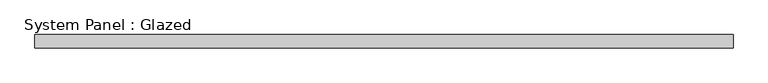
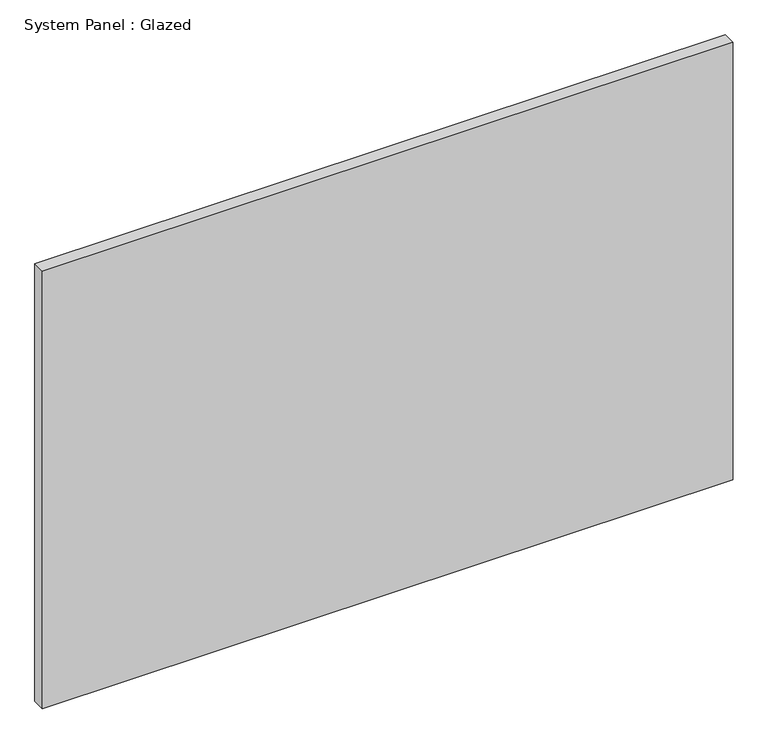
"""IFC4 building model written with IfcOpenShell, lengths in millimetres: plate geometry, System Panel : Glazed."""

from ifc_helpers import new_model, si_unit, origin, origin_with_axes, place, context, project, spatial, polyline, outline, extrude, source, transform, mapped, element, save


def system_panel_glazed_6547e81a(model_context):
    return source(origin(), model_context, "Body", "SweptSolid", [
        extrude(outline(polyline([(669.925, 19.05), (-669.925, 19.05), (-669.925, 44.45), (669.925, 44.45), (669.925, 19.05)])), origin_with_axes(), (0.0, 0.0, 1.0), 897.5064813),
    ])


if __name__ == "__main__":
    model = new_model("IFC4")
    model_context = context("Model", 3, world=origin())
    ifc_project = project(units=[si_unit("LENGTHUNIT", "METRE", prefix="MILLI")], contexts=[model_context])
    site = spatial("IfcSite", under=ifc_project)
    building = spatial("IfcBuilding", under=site)
    placement = place(None, origin())
    system_panel_glazed_shape = system_panel_glazed_6547e81a(model_context)
    element("IfcPlate", 1, ObjectType="System Panel : Glazed", at=placement, inside=building, context=model_context, shape_type="MappedRepresentation", body=[
        mapped(system_panel_glazed_shape, transform((0.0, 0.0, 0.0), x_axis=(1.0, 0.0, 0.0), y_axis=(0.0, 1.0, 0.0), z_axis=(0.0, 0.0, 1.0))),
    ])
    save(model, "model.ifc")

# Revit data of these elements
# Type "System Panel : Glazed"
#   Construction Type Id = "GSP4R"
#   Analytic Construction = "1/8 in Pilkington single glazing"
#   Visual Light Transmittance = 0.9
#   Solar Heat Gain Coefficient = 0.86
#   Heat Transfer Coefficient (U) = 1.18115 BTU/(h·ft²·°F)
#   Define Thermal Properties by = 1
# Element 1 (IfcPlate, "System Panel : Glazed")
#   Materials on its faces: "Glass"
# Materials
#   "Glass": class "Glass", colour RGB 0 128 192, transparency 0.75, Description = "Soda Lime Glass", Cost = 0
